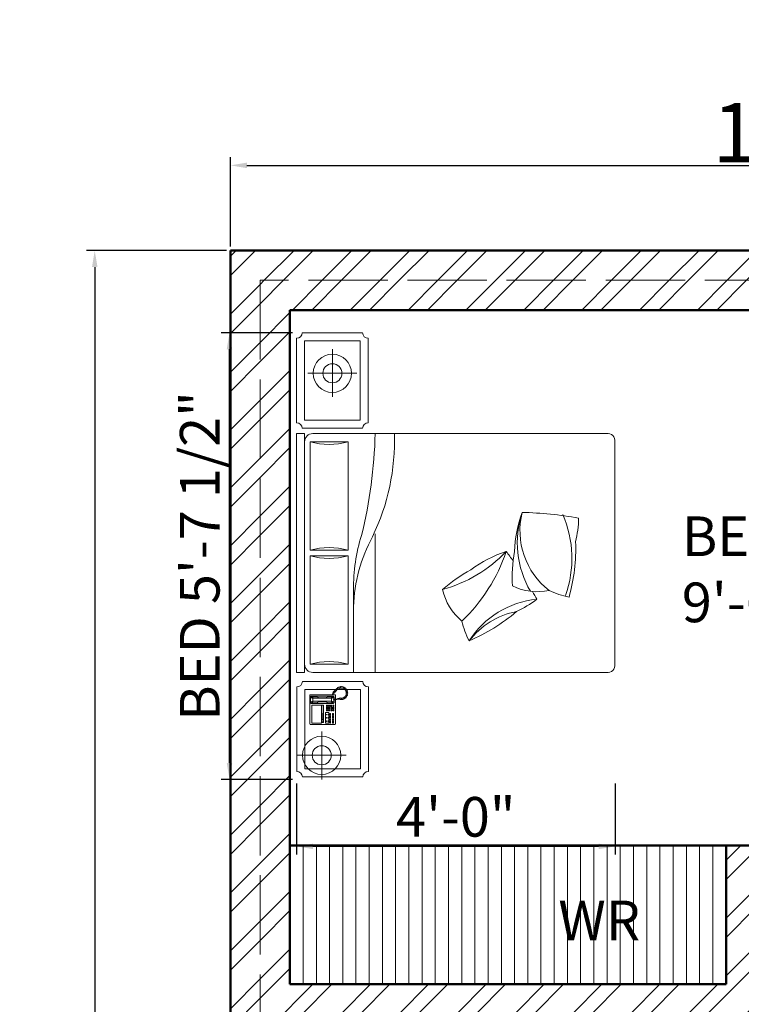
# Model space of a CAD drawing. Units: millimetres. Extents: x 4237 to 5109, y 21391 to 22486.
# Tile 8 of 17: x 4240 to 4349, y 22327 to 22476. Entities that reach past the tile are written whole.
import ezdxf

# ---------------------------------------------------------------- set-up
doc = ezdxf.new("R2010")
doc.units = ezdxf.units.MM
doc.linetypes.add('ACAD_ISO02W100', pattern=[15, 12, -3])
for name, color, linetype, lineweight in [('A-ANNO-DIMS', 2, 'Continuous', 18), ('A-ANNO-TEXT', 7, 'Continuous', 18), ('A-AREA-IDEN', 3, 'Continuous', 18), ('A-FLOR-OVHD', 1, 'ACAD_ISO02W100', 18), ('A-FURN', 8, 'Continuous', 18), ('A-FURN-CASE', 31, 'Continuous', 13), ('A-WALL', 7, 'Continuous', 50), ('A-WALL-PATT', 252, 'Continuous', 13)]:
    doc.layers.add(name, color=color, linetype=linetype, lineweight=lineweight)
doc.styles.get("Standard").update_dxf_attribs({"font": 'arial.ttf'})
doc.dimstyles.new('ISO-25', dxfattribs={"dimtxt": 6, "dimasz": 2.5, "dimexe": 1.25, "dimexo": 0.625, "dimtad": 1, "dimdec": 1, "dimlunit": 4, "dimtxsty": 'Standard', "dimcen": 2.5, "dimadec": 0, "dimazin": 0, "dimtfac": 1, "dimtdec": 1, "dimtmove": 0, "dimatfit": 3, "dimfxl": 1, "dimarcsym": 0})

# ---------------------------------------------------------------- blocks, each defined once
blk = doc.blocks.new('A$C07097A50')
for p, q in [((0.0503, 1.9981), (0.5803, 1.9981)), ((0.1513, 1.6872), (0.1513, 1.9968)), ((0.6716, 1.9489), (0.6716, 2.0001)), ((0.6716, 2.0001), (2.1719, 2.0001)), ((2.1719, 1.9489), (2.1719, 2.0001)), ((2.7701, 1.9993), (2.2401, 1.9993)), ((0.0153, 1.9631), (0.0153, 1.5831)), ((0.0653, 1.9481), (0.0653, 1.5981)), ((0.0653, 1.9481), (0.5653, 1.9481)), ((0.5653, 1.9481), (0.5653, 1.5981)), ((0.6153, 1.9631), (0.6153, 1.5831)), ((2.1719, 1.9489), (0.6716, 1.9489)), ((2.2051, 1.9643), (2.2051, 1.5843)), ((2.2551, 1.9493), (2.2551, 1.5993)), ((2.7551, 1.9493), (2.2551, 1.9493)), ((2.5505, 1.6201), (2.5505, 1.9296)), ((2.7551, 1.9493), (2.7551, 1.5993)), ((2.8051, 1.9643), (2.8051, 1.5843)), ((0.3481, 1.9163), (0.3458, 1.914)), ((0.3458, 1.914), (0.3458, 1.7563)), ((0.3481, 1.9163), (0.5287, 1.9163)), ((0.3526, 1.9037), (0.3526, 1.8431)), ((0.4669, 1.9037), (0.3526, 1.9037)), ((0.4669, 1.8431), (0.4669, 1.9037)), ((0.4772, 1.9071), (0.4818, 1.9129)), ((0.4772, 1.7688), (0.4772, 1.9071)), ((0.4818, 1.9094), (0.4807, 1.9049)), ((0.4807, 1.9049), (0.4807, 1.874)), ((0.4807, 1.9049), (0.4909, 1.8946)), ((0.4807, 1.874), (0.4829, 1.8683)), ((0.4818, 1.9129), (0.5161, 1.9129)), ((0.4864, 1.9117), (0.4818, 1.9094)), ((0.4829, 1.8683), (0.4864, 1.8626)), ((0.4921, 1.8969), (0.4864, 1.9117)), ((0.4864, 1.9117), (0.5138, 1.9117)), ((0.4864, 1.8626), (0.4875, 1.8546)), ((0.4909, 1.8946), (0.4921, 1.8969)), ((0.4909, 1.8431), (0.4909, 1.8946)), ((0.5081, 1.8969), (0.4921, 1.8969)), ((0.5081, 1.8969), (0.5138, 1.9117)), ((0.5092, 1.8946), (0.5081, 1.8969)), ((0.5195, 1.9049), (0.5092, 1.8946)), ((0.5092, 1.8431), (0.5092, 1.8946)), ((0.5138, 1.8626), (0.5127, 1.8546)), ((0.5138, 1.9117), (0.5184, 1.9094)), ((0.5172, 1.8683), (0.5138, 1.8626)), ((0.5161, 1.9129), (0.5218, 1.9071)), ((0.5195, 1.874), (0.5172, 1.8683)), ((0.5184, 1.9094), (0.5195, 1.9049)), ((0.5195, 1.9049), (0.5195, 1.874)), ((0.5218, 1.9071), (0.5218, 1.77)), ((0.5287, 1.9163), (0.5309, 1.914)), ((0.5309, 1.914), (0.5309, 1.7563)), ((0.6716, 1.8977), (0.6716, 0.0512)), ((2.1719, 0.0512), (2.1719, 1.8977)), ((0, 1.8416), (0.3001, 1.8416)), ((0.3526, 1.8431), (0.4669, 1.8431)), ((0.4201, 1.8168), (0.3526, 1.8168)), ((0.3526, 1.8168), (0.3526, 1.7963)), ((0.3526, 1.7963), (0.4201, 1.7963)), ((0.3572, 1.8409), (0.3572, 1.8294)), ((0.4669, 1.8409), (0.3572, 1.8409)), ((0.3572, 1.8294), (0.4669, 1.8294)), ((0.3675, 1.8146), (0.3641, 1.8146)), ((0.3641, 1.8146), (0.3641, 1.8111)), ((0.3641, 1.8111), (0.3675, 1.8111)), ((0.3641, 1.802), (0.3641, 1.7986)), ((0.3675, 1.802), (0.3641, 1.802)), ((0.3641, 1.7986), (0.3675, 1.7986)), ((0.3664, 1.8409), (0.3664, 1.8294)), ((0.3675, 1.8111), (0.3675, 1.8146)), ((0.3675, 1.7986), (0.3675, 1.802)), ((0.3755, 1.8409), (0.3755, 1.8294)), ((0.3846, 1.8409), (0.3846, 1.8294)), ((0.3846, 1.8146), (0.3846, 1.8111)), ((0.3881, 1.8146), (0.3846, 1.8146)), ((0.3846, 1.8111), (0.3881, 1.8111)), ((0.3846, 1.802), (0.3846, 1.7986)), ((0.3881, 1.802), (0.3846, 1.802)), ((0.3846, 1.7986), (0.3881, 1.7986)), ((0.3881, 1.8111), (0.3881, 1.8146)), ((0.3881, 1.7986), (0.3881, 1.802)), ((0.3938, 1.8409), (0.3938, 1.8294)), ((0.4029, 1.8409), (0.4029, 1.8294)), ((0.4052, 1.8146), (0.4052, 1.8111)), ((0.4086, 1.8146), (0.4052, 1.8146)), ((0.4052, 1.8111), (0.4086, 1.8111)), ((0.4052, 1.802), (0.4052, 1.7986)), ((0.4086, 1.802), (0.4052, 1.802)), ((0.4052, 1.7986), (0.4086, 1.7986)), ((0.4086, 1.8111), (0.4086, 1.8146)), ((0.4086, 1.7986), (0.4086, 1.802)), ((0.4121, 1.8409), (0.4121, 1.8294)), ((0.4201, 1.7963), (0.4201, 1.8168)), ((0.4304, 1.8111), (0.4395, 1.8111)), ((0.4304, 1.8043), (0.4304, 1.8111)), ((0.4395, 1.8043), (0.4304, 1.8043)), ((0.4304, 1.7986), (0.4395, 1.7986)), ((0.4304, 1.7917), (0.4304, 1.7986)), ((0.4395, 1.8111), (0.4395, 1.8043)), ((0.4395, 1.7986), (0.4395, 1.7917)), ((0.4441, 1.8043), (0.4441, 1.8111)), ((0.4441, 1.8111), (0.4532, 1.8111)), ((0.4532, 1.8043), (0.4441, 1.8043)), ((0.4441, 1.7986), (0.4532, 1.7986)), ((0.4441, 1.7917), (0.4441, 1.7986)), ((0.4532, 1.8111), (0.4532, 1.8043)), ((0.4532, 1.7986), (0.4532, 1.7917)), ((0.4578, 1.8111), (0.4669, 1.8111)), ((0.4578, 1.8043), (0.4578, 1.8111)), ((0.4669, 1.8043), (0.4578, 1.8043)), ((0.4578, 1.7986), (0.4669, 1.7986)), ((0.4578, 1.7917), (0.4578, 1.7986)), ((0.4669, 1.8294), (0.4669, 1.8409)), ((0.4669, 1.8111), (0.4669, 1.8043)), ((0.4669, 1.7986), (0.4669, 1.7917)), ((0.4807, 1.802), (0.4829, 1.8077)), ((0.4807, 1.7711), (0.4807, 1.802)), ((0.4829, 1.8077), (0.4864, 1.8134)), ((0.4864, 1.8134), (0.4875, 1.8214)), ((0.4875, 1.8546), (0.4875, 1.8431)), ((0.4875, 1.8214), (0.4875, 1.8431)), ((0.4909, 1.8431), (0.4909, 1.7814)), ((0.5092, 1.8431), (0.5092, 1.7814)), ((0.5127, 1.8546), (0.5127, 1.8431)), ((0.5127, 1.8214), (0.5127, 1.8431)), ((0.5138, 1.8134), (0.5127, 1.8214)), ((0.5172, 1.8077), (0.5138, 1.8134)), ((0.5195, 1.802), (0.5172, 1.8077)), ((0.5195, 1.7711), (0.5195, 1.802)), ((0.3458, 1.7563), (0.3481, 1.754)), ((0.5, 1.754), (0.3481, 1.754)), ((0.3652, 1.7906), (0.3538, 1.7906)), ((0.3538, 1.7906), (0.3538, 1.786)), ((0.3538, 1.786), (0.3652, 1.786)), ((0.3538, 1.7666), (0.3538, 1.7734)), ((0.3538, 1.7734), (0.3652, 1.7734)), ((0.3652, 1.7666), (0.3538, 1.7666)), ((0.3652, 1.786), (0.3652, 1.7906)), ((0.3652, 1.7734), (0.3652, 1.7666)), ((0.3812, 1.7906), (0.3698, 1.7906)), ((0.3698, 1.7906), (0.3698, 1.786)), ((0.3698, 1.786), (0.3812, 1.786)), ((0.3698, 1.7666), (0.3698, 1.7734)), ((0.3698, 1.7734), (0.3812, 1.7734)), ((0.3812, 1.7666), (0.3698, 1.7666)), ((0.3812, 1.786), (0.3812, 1.7906)), ((0.3812, 1.7734), (0.3812, 1.7666)), ((0.3972, 1.7906), (0.3858, 1.7906)), ((0.3858, 1.7906), (0.3858, 1.786)), ((0.3858, 1.786), (0.3972, 1.786)), ((0.3858, 1.7666), (0.3858, 1.7734)), ((0.3858, 1.7734), (0.3972, 1.7734)), ((0.3972, 1.7666), (0.3858, 1.7666)), ((0.3972, 1.786), (0.3972, 1.7906)), ((0.3972, 1.7734), (0.3972, 1.7666)), ((0.4018, 1.7906), (0.4018, 1.786)), ((0.4132, 1.7906), (0.4018, 1.7906)), ((0.4018, 1.786), (0.4132, 1.786)), ((0.4018, 1.7734), (0.4132, 1.7734)), ((0.4018, 1.7666), (0.4018, 1.7734)), ((0.4132, 1.7666), (0.4018, 1.7666)), ((0.4132, 1.786), (0.4132, 1.7906)), ((0.4132, 1.7734), (0.4132, 1.7666)), ((0.4395, 1.7917), (0.4304, 1.7917)), ((0.4304, 1.778), (0.4304, 1.7848)), ((0.4304, 1.7848), (0.4395, 1.7848)), ((0.4395, 1.778), (0.4304, 1.778)), ((0.4304, 1.7723), (0.4395, 1.7723)), ((0.4304, 1.7654), (0.4304, 1.7723)), ((0.4395, 1.7654), (0.4304, 1.7654)), ((0.4395, 1.7848), (0.4395, 1.778)), ((0.4395, 1.7723), (0.4395, 1.7654)), ((0.4532, 1.7917), (0.4441, 1.7917)), ((0.4441, 1.778), (0.4441, 1.7848)), ((0.4441, 1.7848), (0.4532, 1.7848)), ((0.4532, 1.778), (0.4441, 1.778)), ((0.4441, 1.7723), (0.4532, 1.7723)), ((0.4441, 1.7654), (0.4441, 1.7723)), ((0.4532, 1.7654), (0.4441, 1.7654)), ((0.4532, 1.7848), (0.4532, 1.778)), ((0.4532, 1.7723), (0.4532, 1.7654)), ((0.4669, 1.7917), (0.4578, 1.7917)), ((0.4578, 1.7791), (0.4578, 1.786)), ((0.4578, 1.786), (0.4669, 1.786)), ((0.4669, 1.7791), (0.4578, 1.7791)), ((0.4578, 1.7654), (0.4578, 1.7723)), ((0.4578, 1.7723), (0.4669, 1.7723)), ((0.4669, 1.7654), (0.4578, 1.7654)), ((0.4669, 1.786), (0.4669, 1.7791)), ((0.4669, 1.7723), (0.4669, 1.7654)), ((0.4829, 1.7631), (0.4772, 1.7688)), ((0.4807, 1.7711), (0.4909, 1.7814)), ((0.4818, 1.7666), (0.4807, 1.7711)), ((0.4864, 1.7643), (0.4818, 1.7666)), ((0.499, 1.7631), (0.4829, 1.7631)), ((0.4921, 1.7791), (0.4864, 1.7643)), ((0.4864, 1.7643), (0.499, 1.7643)), ((0.4909, 1.7814), (0.4921, 1.7791)), ((0.5081, 1.7791), (0.4921, 1.7791)), ((0.5024, 1.7677), (0.4989, 1.7677)), ((0.4989, 1.7677), (0.4991, 1.7578)), ((0.4991, 1.7578), (0.5019, 1.7463)), ((0.5019, 1.7463), (0.5047, 1.7354)), ((0.503, 1.7585), (0.5024, 1.7677)), ((0.5026, 1.7643), (0.5138, 1.7643)), ((0.5161, 1.7631), (0.5027, 1.7631)), ((0.5047, 1.7511), (0.503, 1.7585)), ((0.5287, 1.754), (0.504, 1.754)), ((0.5047, 1.7354), (0.5044, 1.7294)), ((0.5074, 1.7403), (0.5047, 1.7511)), ((0.5081, 1.7347), (0.5074, 1.7403)), ((0.5079, 1.7287), (0.5081, 1.7347)), ((0.5092, 1.7814), (0.5081, 1.7791)), ((0.5081, 1.7791), (0.5138, 1.7643)), ((0.5195, 1.7711), (0.5092, 1.7814)), ((0.5138, 1.7643), (0.5184, 1.7666)), ((0.5218, 1.77), (0.5161, 1.7631)), ((0.5184, 1.7666), (0.5195, 1.7711)), ((0.5309, 1.7563), (0.5287, 1.754)), ((0.5378, 1.7743), (0.5309, 1.7768)), ((0.5309, 1.7723), (0.536, 1.7709)), ((0.536, 1.7709), (0.5406, 1.7672)), ((0.541, 1.7711), (0.5378, 1.7743)), ((0.5406, 1.7672), (0.5418, 1.7656)), ((0.5434, 1.7689), (0.541, 1.7711)), ((0.5442, 1.7658), (0.5418, 1.7634)), ((0.5418, 1.7656), (0.5442, 1.7658)), ((0.5418, 1.7634), (0.5511, 1.7552)), ((0.5477, 1.7705), (0.5434, 1.7689)), ((0.5497, 1.7685), (0.5477, 1.7705)), ((0.5481, 1.765), (0.5497, 1.7685)), ((0.5509, 1.7672), (0.5481, 1.765)), ((0.5539, 1.764), (0.5509, 1.7672)), ((0.5511, 1.7552), (0.5662, 1.7423)), ((0.5515, 1.7574), (0.5539, 1.764)), ((0.5577, 1.7606), (0.5515, 1.7574)), ((0.563, 1.7556), (0.5577, 1.7606)), ((0.5618, 1.7483), (0.563, 1.7556)), ((0.567, 1.7515), (0.5618, 1.7483)), ((0.5664, 1.7419), (0.574, 1.7201)), ((0.5714, 1.7469), (0.567, 1.7515)), ((0.5696, 1.7419), (0.5714, 1.7469)), ((0.5766, 1.7426), (0.5697, 1.7419)), ((0.572, 1.7331), (0.5787, 1.7356)), ((0.5794, 1.7333), (0.572, 1.7331)), ((0.5787, 1.7356), (0.5766, 1.7426)), ((0.581, 1.728), (0.5794, 1.7333)), ((2.7018, 1.7745), (2.4017, 1.7745)), ((0.5026, 1.7254), (0.5021, 1.7199)), ((0.5021, 1.7199), (0.5088, 1.7187)), ((0.5088, 1.7187), (0.5023, 1.7148)), ((0.5023, 1.7148), (0.5028, 1.7085)), ((0.5051, 1.728), (0.5026, 1.7254)), ((0.5028, 1.7085), (0.5102, 1.7078)), ((0.5102, 1.7078), (0.5037, 1.7028)), ((0.5037, 1.7028), (0.5067, 1.6974)), ((0.5044, 1.7294), (0.5051, 1.728)), ((0.5067, 1.6974), (0.5137, 1.6988)), ((0.5121, 1.7257), (0.5079, 1.7287)), ((0.5137, 1.6988), (0.5104, 1.6923)), ((0.5104, 1.6923), (0.5139, 1.6882)), ((0.5111, 1.7203), (0.5121, 1.7257)), ((0.5123, 1.7058), (0.5111, 1.7203)), ((0.5211, 1.6947), (0.5123, 1.7058)), ((0.5139, 1.6882), (0.5192, 1.6921)), ((0.5192, 1.6921), (0.5183, 1.6859)), ((0.5183, 1.6859), (0.5227, 1.6831)), ((0.5333, 1.6882), (0.5211, 1.6947)), ((0.5227, 1.6831), (0.5282, 1.6877)), ((0.5282, 1.6877), (0.5276, 1.6801)), ((0.5276, 1.6801), (0.5324, 1.6787)), ((0.5324, 1.6787), (0.5354, 1.6849)), ((0.5472, 1.687), (0.5333, 1.6882)), ((0.5354, 1.6849), (0.5382, 1.6787)), ((0.5382, 1.6787), (0.5421, 1.6782)), ((0.5421, 1.6782), (0.5437, 1.6849)), ((0.5437, 1.6849), (0.5463, 1.6775)), ((0.5463, 1.6775), (0.5507, 1.6787)), ((0.5606, 1.6928), (0.5472, 1.687)), ((0.5507, 1.6787), (0.5509, 1.6849)), ((0.5509, 1.6849), (0.5562, 1.6803)), ((0.5562, 1.6803), (0.5599, 1.6822)), ((0.5592, 1.6891), (0.5641, 1.6831)), ((0.5599, 1.6822), (0.5592, 1.6891)), ((0.5708, 1.7028), (0.5606, 1.6928)), ((0.5641, 1.6831), (0.5678, 1.6863)), ((0.565, 1.6926), (0.5715, 1.6898)), ((0.5678, 1.6863), (0.565, 1.6926)), ((0.574, 1.7201), (0.5708, 1.7028)), ((0.5745, 1.6926), (0.5713, 1.6988)), ((0.5713, 1.6988), (0.578, 1.6967)), ((0.5715, 1.6898), (0.5745, 1.6926)), ((0.5743, 1.7076), (0.5814, 1.7074)), ((0.5798, 1.7014), (0.5743, 1.7076)), ((0.5761, 1.7234), (0.581, 1.728)), ((0.5824, 1.7234), (0.5761, 1.7234)), ((0.5764, 1.7155), (0.5835, 1.7176)), ((0.5824, 1.712), (0.5764, 1.7155)), ((0.578, 1.6967), (0.5798, 1.7014)), ((0.5814, 1.7074), (0.5824, 1.712)), ((0.5835, 1.7176), (0.5824, 1.7234)), ((0.0503, 1.5481), (0.5803, 1.5481)), ((0.0653, 1.5981), (0.5653, 1.5981)), ((2.7701, 1.5493), (2.2401, 1.5493)), ((2.7551, 1.5993), (2.2551, 1.5993)), ((0.7228, 0.0001), (2.1207, 0.0001))]:
    blk.add_line(p, q)
at = {"linetype": 'ByBlock'}
for p, q in [((0.7228, 1.6759), (0.7228, 1.9148)), ((0.7228, 1.9148), (1.4047, 1.9148)), ((1.4047, 1.9148), (1.4047, 1.6759)), ((1.4388, 1.6759), (1.4388, 1.9148)), ((1.4388, 1.9148), (2.1207, 1.9148)), ((2.1207, 1.9148), (2.1207, 1.6759)), ((1.4047, 1.6759), (0.7228, 1.6759)), ((2.1207, 1.6759), (1.4388, 1.6759)), ((1.1914, 1.6418), (0.6716, 1.6418)), ((1.5412, 1.5053), (0.6716, 1.5053))]:
    blk.add_line(p, q, dxfattribs=at)
for centre in [(0.1513, 1.8416), (2.5505, 1.7745)]:
    blk.add_circle(centre, 0.12, dxfattribs=at)
for centre in [(0.1513, 1.8416), (2.5505, 1.7745)]:
    blk.add_circle(centre, 0.06)
for centre, radius, start, end in [((0.0153, 1.9981), 0.035, 270, 0), ((0.6153, 1.9981), 0.035, 180, 270), ((2.2051, 1.9993), 0.035, 270, 0), ((2.8051, 1.9993), 0.035, 180, 270), ((0.7228, 1.8977), 0.0512, 90, 180), ((2.1207, 1.8977), 0.0512, 0, 90), ((0.0153, 1.5481), 0.035, 0, 90), ((0.6153, 1.5481), 0.035, 90, 180), ((2.2051, 1.5493), 0.035, 0, 90), ((2.8051, 1.5493), 0.035, 90, 180), ((1.2698, 0.7333), 0.3575, 102.47819, 140.46254), ((0.4476, 0.4335), 0.9879, 28.49711, 41.05657), ((2.0313, 1.3124), 0.8697, 195.33601, 226.41927), ((1.1192, 0.4274), 0.548, 103.20343, 117.03623), ((1.7756, 1.7059), 1.0798, 223.63057, 251.4288), ((1.9422, 1.372), 1.1652, 203.06416, 220.32086), ((0.5744, 0.5274), 0.4879, 10.69865, 52.68638), ((0.5678, 0.4375), 0.5655, 5.33912, 57.68949), ((0.6844, 0.4345), 0.7874, 18.35266, 36.68512), ((0.1017, 2.4319), 2.1977, 305.29657, 307.24182), ((1.5362, 0.487), 0.3575, 154.0418, 192.02615), ((1.2599, -0.3434), 0.9879, 80.06073, 92.62018), ((1.4063, -0.1573), 0.7874, 69.91627, 88.24873), ((1.7177, 0.9312), 0.734, 205.25901, 216.93514), ((1.4868, 0.0041), 0.6085, 71.81005, 120.13512), ((1.5627, 0.1186), 0.4774, 76.18494, 142.00166), ((-0.5205, 0.628), 2.1977, 349.48843, 358.80544), ((0.1017, 2.4319), 2.1977, 297.92482, 299.3793), ((1.6822, 0.1789), 0.548, 154.76704, 168.59984), ((1.3874, 0.9578), 0.6885, 250.29361, 293.6414), ((1.4539, 1.4107), 1.1652, 254.62778, 271.88448), ((1.6595, 0.9609), 0.734, 256.82263, 268.49876), ((0.717, 0.0455), 0.0458, 172.75992, 277.24008), ((2.1265, 0.0455), 0.0458, 262.75992, 7.24008)]:
    blk.add_arc(centre, radius, start, end)
for centre, radius, start, end in [((0.3133, 1.7953), 0.4265, 343.73979, 16.26021), ((1.8141, 1.7953), 0.4265, 163.73979, 196.26021), ((1.0294, 1.7953), 0.4265, 343.73979, 16.26021), ((2.5302, 1.7953), 0.4265, 163.73979, 196.26021), ((1.053, 0.6571), 0.9853, 61.43285, 88.12613), ((1.2053, 0.5713), 1.0706, 72.19663, 90.74184), ((2.2595, 4.5996), 3.0955, 256.42012, 268.37887), ((2.1283, 2.7745), 1.3903, 244.24266, 271.79845)]:
    blk.add_arc(centre, radius, start, end, dxfattribs=at)
blk = doc.blocks.new('*D56')
at = {"layer": 'A-ANNO-DIMS', "color": 0, "lineweight": -2, "transparency": 16777216}
for p, q in [((4271.65, 22441.33), (4271.65, 22454.84)), ((4458.3, 22441.33), (4458.3, 22454.84)), ((4274.15, 22453.59), (4455.8, 22453.59))]:
    blk.add_line(p, q, dxfattribs=at)
at = {"layer": 'A-ANNO-DIMS', "color": 0, "transparency": 16777216}
for points in [[(4274.15, 22454.01), (4274.15, 22453.17), (4271.65, 22453.59)], [(4455.8, 22454.01), (4455.8, 22453.17), (4458.3, 22453.59)]]:
    blk.add_solid(points, dxfattribs=at)
at = {"layer": 'Defpoints', "color": 0, "transparency": 16777216}
for p in [(4458.3, 22453.59), (4271.65, 22440.7), (4458.3, 22440.7)]:
    blk.add_point(p, dxfattribs=at)
at = {"layer": 'A-ANNO-DIMS', "color": 0, "transparency": 16777216, "insert": (4364.98, 22464.83), "char_height": 9, "attachment_point": 5}
blk.add_mtext('15\'-6{\\H1x;\\S1/2;}"', dxfattribs=at)
blk = doc.blocks.new('*D58')
at = {"layer": 'A-ANNO-DIMS', "color": 0, "lineweight": -2, "transparency": 16777216}
for p, q in [((4271.03, 22440.7), (4249.86, 22440.7)), ((4251.11, 22438.2), (4251.11, 22035.2)), ((4271.03, 22032.7), (4249.86, 22032.7))]:
    blk.add_line(p, q, dxfattribs=at)
at = {"layer": 'A-ANNO-DIMS', "color": 0, "transparency": 16777216}
for points in [[(4250.69, 22438.2), (4251.53, 22438.2), (4251.11, 22440.7)], [(4250.69, 22035.2), (4251.53, 22035.2), (4251.11, 22032.7)]]:
    blk.add_solid(points, dxfattribs=at)
at = {"layer": 'Defpoints', "color": 0, "transparency": 16777216}
for p in [(4271.65, 22440.7), (4251.11, 22032.7), (4271.65, 22032.7)]:
    blk.add_point(p, dxfattribs=at)
at = {"layer": 'A-ANNO-DIMS', "color": 0, "transparency": 16777216, "insert": (4245.89, 22236.7), "char_height": 9, "attachment_point": 5, "rotation": 90}
blk.add_mtext("34'", dxfattribs=at)
blk = doc.blocks.new('*D64')
at = {"layer": 'A-ANNO-DIMS', "color": 0, "lineweight": -2, "transparency": 16777216}
for p, q in [((4281.02, 22428.27), (4270.26, 22428.27)), ((4271.51, 22363.2), (4271.51, 22425.77)), ((4281.02, 22360.7), (4270.26, 22360.7))]:
    blk.add_line(p, q, dxfattribs=at)
at = {"layer": 'A-ANNO-DIMS', "color": 0, "transparency": 16777216}
for points in [[(4271.09, 22425.77), (4271.92, 22425.77), (4271.51, 22428.27)], [(4271.09, 22363.2), (4271.92, 22363.2), (4271.51, 22360.7)]]:
    blk.add_solid(points, dxfattribs=at)
at = {"layer": 'Defpoints', "color": 0, "transparency": 16777216}
for p in [(4271.51, 22428.27), (4281.64, 22428.27), (4281.64, 22360.7)]:
    blk.add_point(p, dxfattribs=at)
at = {"layer": 'A-ANNO-DIMS', "color": 0, "transparency": 16777216, "insert": (4267.78, 22394.49), "char_height": 6, "attachment_point": 5, "rotation": 90}
blk.add_mtext('BED 5\'-7 1/2"', dxfattribs=at)
blk = doc.blocks.new('*D65')
at = {"layer": 'A-ANNO-DIMS', "color": 0, "lineweight": -2, "transparency": 16777216}
for p, q in [((4281.64, 22360.08), (4281.64, 22349.32)), ((4329.86, 22360.08), (4329.86, 22349.32)), ((4327.36, 22350.57), (4284.14, 22350.57))]:
    blk.add_line(p, q, dxfattribs=at)
at = {"layer": 'A-ANNO-DIMS', "color": 0, "transparency": 16777216}
for points in [[(4284.14, 22350.98), (4284.14, 22350.15), (4281.64, 22350.57)], [(4327.36, 22350.98), (4327.36, 22350.15), (4329.86, 22350.57)]]:
    blk.add_solid(points, dxfattribs=at)
at = {"layer": 'Defpoints', "color": 0, "transparency": 16777216}
for p in [(4281.64, 22360.7), (4329.86, 22360.7), (4281.64, 22350.57)]:
    blk.add_point(p, dxfattribs=at)
at = {"layer": 'A-ANNO-DIMS', "color": 0, "transparency": 16777216, "insert": (4305.75, 22354.26), "char_height": 6, "attachment_point": 5}
blk.add_mtext('4\'-0"', dxfattribs=at)

msp = doc.modelspace()

# ---------------------------------------------------------------- hatches: boundary and pattern name
at = {"layer": 'A-WALL-PATT'}
h = msp.add_hatch(dxfattribs=at)
h.set_pattern_fill('ANSI32', color=256, scale=0.65)
h.paths.add_polyline_path([(4399.15, 22440.7), (4271.65, 22440.7), (4271.65, 22032.7), (4276.15, 22032.7), (4276.15, 22044.7), (4276.15, 22436.2), (4399.15, 22436.2)])
h.paths.add_polyline_path([(4351.15, 22185.7), (4357.15, 22185.7), (4357.15, 22194.7), (4346.65, 22194.7), (4346.65, 22080.7), (4351.15, 22080.7)], flags=16)
h.paths.add_polyline_path([(4351.15, 22295.2), (4346.65, 22295.2), (4346.65, 22238.2), (4311.53, 22238.2), (4311.53, 22233.7), (4351.15, 22233.7)], flags=16)
h = msp.add_hatch(dxfattribs=at)
h.set_pattern_fill('ANSI32', color=256, scale=0.65)
h.paths.add_polyline_path([(4399.15, 22436.2), (4276.15, 22436.2), (4276.15, 22044.7), (4280.65, 22044.7), (4280.65, 22233.7), (4287.73, 22233.7), (4287.73, 22238.2), (4280.65, 22238.2), (4280.65, 22325.2), (4351.15, 22325.2), (4351.15, 22350.7), (4346.65, 22350.7), (4346.65, 22329.7), (4280.65, 22329.7), (4280.65, 22431.7), (4394.65, 22431.7), (4399.15, 22431.7)], flags=17)
h.paths.add_polyline_path([(4351.15, 22185.7), (4357.15, 22185.7), (4357.15, 22194.7), (4346.65, 22194.7), (4346.65, 22080.7), (4351.15, 22080.7)], flags=16)
h.paths.add_polyline_path([(4351.15, 22295.2), (4346.65, 22295.2), (4346.65, 22238.2), (4311.53, 22238.2), (4311.53, 22233.7), (4351.15, 22233.7)], flags=16)

# ---------------------------------------------------------------- linework, layer by layer
at = {"layer": 'A-FLOR-OVHD'}
msp.add_lwpolyline([(4640.45, 22032.7), (4640.45, 22436.2), (4276.15, 22436.2), (4276.15, 22032.7)], dxfattribs=at)
at = {"layer": 'A-FURN-CASE'}
for p, q in [((4282.65, 22329.7), (4282.65, 22350.7)), ((4284.65, 22329.7), (4284.65, 22350.7)), ((4286.65, 22329.7), (4286.65, 22350.7)), ((4288.65, 22329.7), (4288.65, 22350.7)), ((4290.65, 22329.7), (4290.65, 22350.7)), ((4292.65, 22329.7), (4292.65, 22350.7)), ((4294.65, 22329.7), (4294.65, 22350.7)), ((4296.65, 22329.7), (4296.65, 22350.7)), ((4298.65, 22329.7), (4298.65, 22350.7)), ((4300.65, 22329.7), (4300.65, 22350.7)), ((4302.65, 22329.7), (4302.65, 22350.7)), ((4304.65, 22329.7), (4304.65, 22350.7)), ((4306.65, 22329.7), (4306.65, 22350.7)), ((4308.65, 22329.7), (4308.65, 22350.7)), ((4310.65, 22329.7), (4310.65, 22350.7)), ((4312.65, 22329.7), (4312.65, 22350.7)), ((4314.65, 22329.7), (4314.65, 22350.7)), ((4316.65, 22329.7), (4316.65, 22350.7)), ((4318.65, 22329.7), (4318.65, 22350.7)), ((4320.65, 22329.7), (4320.65, 22350.7)), ((4322.65, 22329.7), (4322.65, 22350.7)), ((4324.65, 22329.7), (4324.65, 22350.7)), ((4326.65, 22329.7), (4326.65, 22350.7)), ((4328.65, 22329.7), (4328.65, 22350.7)), ((4330.65, 22329.7), (4330.65, 22350.7)), ((4332.65, 22329.7), (4332.65, 22350.7)), ((4334.65, 22329.7), (4334.65, 22350.7)), ((4336.65, 22329.7), (4336.65, 22350.7)), ((4338.65, 22329.7), (4338.65, 22350.7)), ((4340.65, 22329.7), (4340.65, 22350.7)), ((4342.65, 22329.7), (4342.65, 22350.7)), ((4344.65, 22329.7), (4344.65, 22350.7))]:
    msp.add_line(p, q, dxfattribs=at)
at = {"layer": 'A-WALL'}
for p, q in [((4271.65, 22440.7), (4271.65, 22032.7)), ((4271.65, 22440.7), (4644.95, 22440.7)), ((4280.65, 22431.7), (4280.65, 22329.7)), ((4280.65, 22431.7), (4394.65, 22431.7)), ((4280.65, 22350.7), (4351.15, 22350.7)), ((4346.65, 22329.7), (4346.65, 22350.7)), ((4280.65, 22329.7), (4346.65, 22329.7))]:
    msp.add_line(p, q, dxfattribs=at)

# ---------------------------------------------------------------- block references
at = {"layer": 'A-FURN', "xscale": 24.08776378444, "yscale": 24.08776378444, "zscale": 24.08776378444, "rotation": 90}
msp.add_blockref('A$C07097A50', (4329.82, 22360.7), dxfattribs=at)

# ---------------------------------------------------------------- texts
at = {"layer": 'A-ANNO-TEXT', "insert": (4315.77, 22342.36), "char_height": 6, "attachment_point": 1}
msp.add_mtext_dynamic_manual_height_columns('   WR', width=21.7253, gutter_width=12.5, heights=[0], dxfattribs=at)
at = {"layer": 'A-AREA-IDEN', "insert": (4339.96, 22400.48), "char_height": 6, "attachment_point": 1}
msp.add_mtext_dynamic_manual_height_columns('BED ROOM \\P9\'-6\' X 8\'-6"', width=55.7646, gutter_width=12.5, heights=[0], dxfattribs=at)

# ---------------------------------------------------------------- dimensions: what is measured, and where the dimension line sits
at = {"layer": 'A-ANNO-DIMS'}
dim = msp.add_linear_dim(base=(4458.30138825, 22453.59015802), p1=(4271.65138825, 22440.70062861), p2=(4458.30138825, 22440.70062861), dimstyle='ISO-25', override={"dimtxt": 9, "dimclrd": 0, "dimclre": 0, "dimclrt": 0}, dxfattribs=at)
dim.commit()
dim.dimension.update_dxf_attribs({"geometry": '*D56', "text_midpoint": (4364.97638825, 22464.82873237)})
for base, p1, p2, angle, override, picture, middle in [((4251.11, 22032.7), (4271.65, 22440.7), (4271.65, 22032.7), 90, {"dimtxt": 9, "dimclrd": 0, "dimclre": 0, "dimclrt": 0}, '*D58', (4245.89, 22236.7)), ((4281.64, 22350.57), (4329.86, 22360.7), (4281.64, 22360.7), 180, {"dimdec": 1, "dimrnd": 0, "dimzin": 1, "dimlunit": 4, "dimfrac": 2}, '*D65', (4305.75, 22354.26))]:
    dim = msp.add_linear_dim(base=base, p1=p1, p2=p2, angle=angle, dimstyle='ISO-25', override=override, dxfattribs=at)
    dim.commit()
    dim.dimension.update_dxf_attribs({"geometry": picture, "text_midpoint": middle})
dim = msp.add_linear_dim(base=(4271.51, 22428.27), p1=(4281.64, 22360.7), p2=(4281.64, 22428.27), angle=90, text='BED <>', dimstyle='ISO-25', override={"dimdec": 1, "dimrnd": 0, "dimzin": 1, "dimlunit": 4, "dimfrac": 2}, dxfattribs=at)
dim.commit()
dim.dimension.update_dxf_attribs({"geometry": '*D64', "text_midpoint": (4267.78, 22394.49)})

doc.saveas('drawing.dxf')
